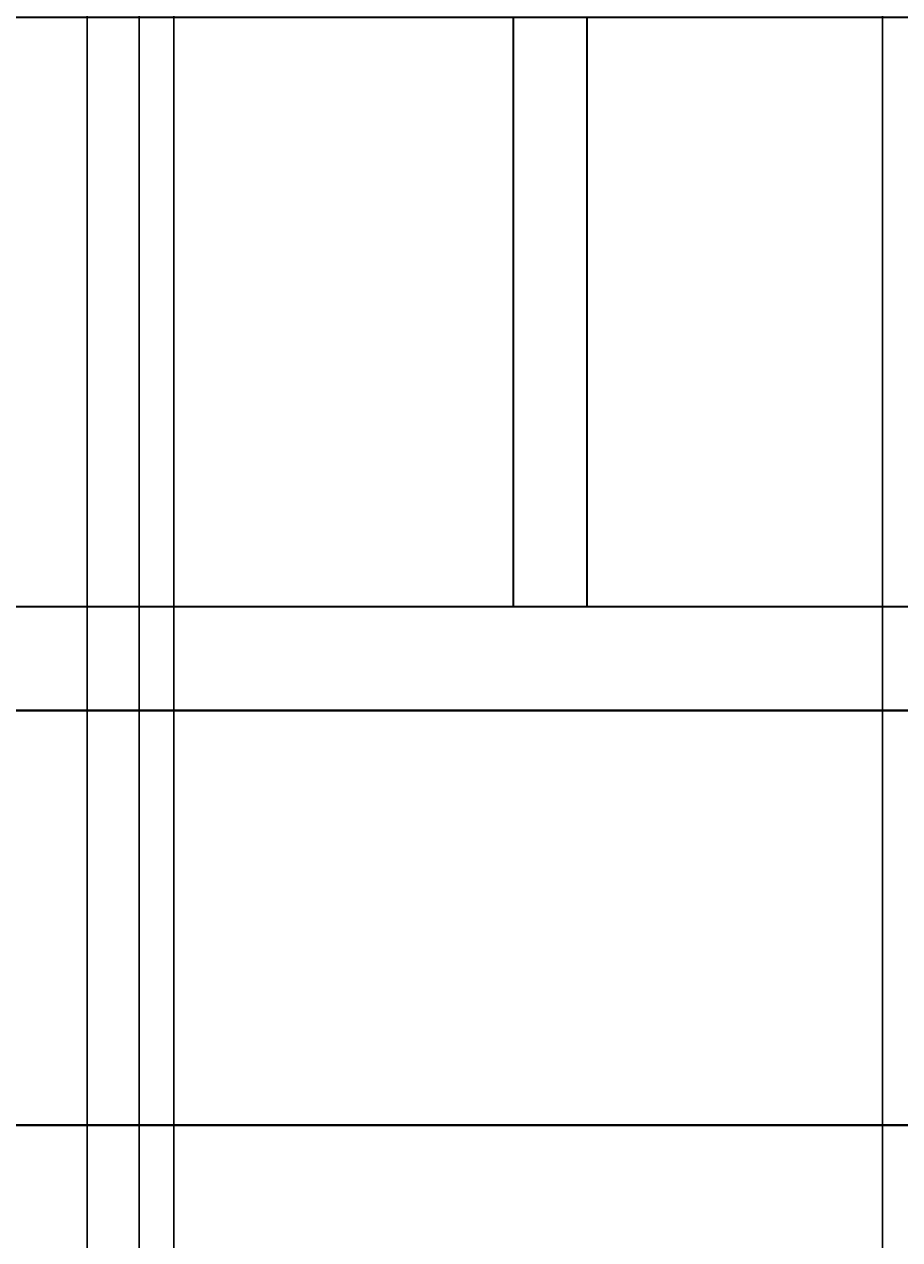
# Model space of a CAD drawing. Units: inches. Extents: x -6 to 289, y -8 to 323.
# Tile 62 of 107: x 186 to 212, y 124 to 159. Entities that reach past the tile are written whole.
import ezdxf

# ---------------------------------------------------------------- set-up
doc = ezdxf.new("R2010")
doc.units = ezdxf.units.IN
doc.header["$MEASUREMENT"] = 0
doc.layers.add('A-ANNO-DIMS', color=2, linetype='Continuous', lineweight=18)
doc.layers.add('A-ELEV', color=7, linetype='Continuous', lineweight=35)
doc.styles.get("Standard").update_dxf_attribs({"font": 'arial.ttf'})
doc.dimstyles.get("Standard").update_dxf_attribs({"dimtxt": 0.18, "dimasz": 0.18, "dimexe": 0.18, "dimexo": 0.0625, "dimgap": 0.09, "dimtad": 0, "dimtih": 1, "dimtoh": 1, "dimdec": 4, "dimzin": 0, "dimdsep": 46, "dimtxsty": 'Standard', "dimcen": 0.09, "dimadec": 0, "dimazin": 0, "dimtfac": 1, "dimtdec": 4, "dimtofl": 0, "dimtmove": 0, "dimatfit": 3, "dimfxl": 1, "dimtolj": 1, "dimtzin": 0, "dimarcsym": 0})

# ---------------------------------------------------------------- blocks, each defined once
blk = doc.blocks.new('*D24')
at = {"layer": 'A-ANNO-DIMS', "color": 0, "lineweight": -2, "transparency": 16777216}
for p, q in [((126.946, 178.654), (288.653, 178.654)), ((288.473, 178.474), (288.473, 159.153)), ((288.473, 139.469), (288.473, 158.789)), ((259.226, 139.289), (288.653, 139.289))]:
    blk.add_line(p, q, dxfattribs=at)
at = {"layer": 'A-ANNO-DIMS', "color": 0, "transparency": 16777216}
for points in [[(288.443, 178.474), (288.503, 178.474), (288.473, 178.654)], [(288.443, 139.469), (288.503, 139.469), (288.473, 139.289)]]:
    blk.add_solid(points, dxfattribs=at)
at = {"layer": 'Defpoints', "color": 0, "transparency": 16777216}
for p in [(126.883, 178.654), (288.473, 178.654), (259.164, 139.289)]:
    blk.add_point(p, dxfattribs=at)
at = {"layer": 'A-ANNO-DIMS', "color": 0, "transparency": 16777216, "insert": (288.473, 158.971), "char_height": 0.18, "attachment_point": 5}
blk.add_mtext('\\A1;39.365', dxfattribs=at)
blk = doc.blocks.new('*D40')
at = {"layer": 'A-ANNO-DIMS', "color": 0, "lineweight": -2, "transparency": 16777216}
for p, q in [((188.292, 226.826), (188.292, -8.391)), ((189.792, 225.326), (189.792, -8.391)), ((188.472, -8.211), (188.796, -8.211)), ((189.612, -8.211), (189.288, -8.211))]:
    blk.add_line(p, q, dxfattribs=at)
at = {"layer": 'A-ANNO-DIMS', "color": 0, "transparency": 16777216}
for points in [[(188.472, -8.181), (188.472, -8.241), (188.292, -8.211)], [(189.612, -8.181), (189.612, -8.241), (189.792, -8.211)]]:
    blk.add_solid(points, dxfattribs=at)
at = {"layer": 'Defpoints', "color": 0, "transparency": 16777216}
for p in [(188.292, 226.889), (189.792, 225.389), (189.792, -8.211)]:
    blk.add_point(p, dxfattribs=at)
at = {"layer": 'A-ANNO-DIMS', "color": 0, "transparency": 16777216, "insert": (189.042, -8.211), "char_height": 0.18, "attachment_point": 5}
blk.add_mtext('\\A1;1.5', dxfattribs=at)
blk = doc.blocks.new('*D41')
at = {"layer": 'A-ANNO-DIMS', "color": 0, "lineweight": -2, "transparency": 16777216}
for p, q in [((189.792, 225.326), (189.792, -8.391)), ((190.792, 224.326), (190.792, -8.391)), ((189.972, -8.211), (190.169, -8.211)), ((190.612, -8.211), (190.415, -8.211))]:
    blk.add_line(p, q, dxfattribs=at)
at = {"layer": 'A-ANNO-DIMS', "color": 0, "transparency": 16777216}
for points in [[(189.972, -8.181), (189.972, -8.241), (189.792, -8.211)], [(190.612, -8.181), (190.612, -8.241), (190.792, -8.211)]]:
    blk.add_solid(points, dxfattribs=at)
at = {"layer": 'Defpoints', "color": 0, "transparency": 16777216}
for p in [(189.792, 225.389), (190.792, 224.389), (190.792, -8.211)]:
    blk.add_point(p, dxfattribs=at)
at = {"layer": 'A-ANNO-DIMS', "color": 0, "transparency": 16777216, "insert": (190.292, -8.211), "char_height": 0.18, "attachment_point": 5}
blk.add_mtext('\\A1;1', dxfattribs=at)
blk = doc.blocks.new('*D42')
at = {"layer": 'A-ANNO-DIMS', "color": 0, "lineweight": -2, "transparency": 16777216}
for p, q in [((190.792, 224.326), (190.792, -8.391)), ((211.292, 224.326), (211.292, -8.391)), ((190.972, -8.211), (200.716, -8.211)), ((211.112, -8.211), (201.368, -8.211))]:
    blk.add_line(p, q, dxfattribs=at)
at = {"layer": 'A-ANNO-DIMS', "color": 0, "transparency": 16777216}
for points in [[(190.972, -8.181), (190.972, -8.241), (190.792, -8.211)], [(211.112, -8.181), (211.112, -8.241), (211.292, -8.211)]]:
    blk.add_solid(points, dxfattribs=at)
at = {"layer": 'Defpoints', "color": 0, "transparency": 16777216}
for p in [(190.792, 224.389), (211.292, 224.389), (211.292, -8.211)]:
    blk.add_point(p, dxfattribs=at)
at = {"layer": 'A-ANNO-DIMS', "color": 0, "transparency": 16777216, "insert": (201.042, -8.211), "char_height": 0.18, "attachment_point": 5}
blk.add_mtext('\\A1;20.5', dxfattribs=at)
blk = doc.blocks.new('*D43')
at = {"layer": 'A-ANNO-DIMS', "color": 0, "lineweight": -2, "transparency": 16777216}
for p, q in [((211.292, 224.326), (211.292, -8.391)), ((212.292, 224.326), (212.292, -8.391)), ((211.472, -8.211), (211.669, -8.211)), ((212.112, -8.211), (211.915, -8.211))]:
    blk.add_line(p, q, dxfattribs=at)
at = {"layer": 'A-ANNO-DIMS', "color": 0, "transparency": 16777216}
for points in [[(211.472, -8.181), (211.472, -8.241), (211.292, -8.211)], [(212.112, -8.181), (212.112, -8.241), (212.292, -8.211)]]:
    blk.add_solid(points, dxfattribs=at)
at = {"layer": 'Defpoints', "color": 0, "transparency": 16777216}
for p in [(211.292, 224.389), (212.292, 224.389), (212.292, -8.211)]:
    blk.add_point(p, dxfattribs=at)
at = {"layer": 'A-ANNO-DIMS', "color": 0, "transparency": 16777216, "insert": (211.792, -8.211), "char_height": 0.18, "attachment_point": 5}
blk.add_mtext('\\A1;1', dxfattribs=at)
blk = doc.blocks.new('*D79')
at = {"layer": 'A-ANNO-DIMS', "color": 0, "lineweight": -2, "transparency": 16777216}
for p, q in [((171.296, 118.033), (171.296, 322.969)), ((188.292, 116.842), (188.292, 322.969)), ((171.476, 322.789), (179.339, 322.789)), ((188.112, 322.789), (180.249, 322.789))]:
    blk.add_line(p, q, dxfattribs=at)
at = {"layer": 'A-ANNO-DIMS', "color": 0, "transparency": 16777216}
for points in [[(171.476, 322.819), (171.476, 322.759), (171.296, 322.789)], [(188.112, 322.819), (188.112, 322.759), (188.292, 322.789)]]:
    blk.add_solid(points, dxfattribs=at)
at = {"layer": 'Defpoints', "color": 0, "transparency": 16777216}
for p in [(188.292, 322.789), (171.296, 117.971), (188.292, 116.779)]:
    blk.add_point(p, dxfattribs=at)
at = {"layer": 'A-ANNO-DIMS', "color": 0, "transparency": 16777216, "insert": (179.794, 322.789), "char_height": 0.18, "attachment_point": 5}
blk.add_mtext('\\A1;16.996', dxfattribs=at)
blk = doc.blocks.new('*D80')
at = {"layer": 'A-ANNO-DIMS', "color": 0, "lineweight": -2, "transparency": 16777216}
for p, q in [((188.292, 116.842), (188.292, 322.969)), ((230.292, 116.842), (230.292, 322.969)), ((188.472, 322.789), (209.07, 322.789)), ((230.112, 322.789), (209.513, 322.789))]:
    blk.add_line(p, q, dxfattribs=at)
at = {"layer": 'A-ANNO-DIMS', "color": 0, "transparency": 16777216}
for points in [[(188.472, 322.819), (188.472, 322.759), (188.292, 322.789)], [(230.112, 322.819), (230.112, 322.759), (230.292, 322.789)]]:
    blk.add_solid(points, dxfattribs=at)
at = {"layer": 'Defpoints', "color": 0, "transparency": 16777216}
for p in [(230.292, 322.789), (188.292, 116.779), (230.292, 116.779)]:
    blk.add_point(p, dxfattribs=at)
at = {"layer": 'A-ANNO-DIMS', "color": 0, "transparency": 16777216, "insert": (209.292, 322.789), "char_height": 0.18, "attachment_point": 5}
blk.add_mtext('\\A1;42', dxfattribs=at)

msp = doc.modelspace()

# ---------------------------------------------------------------- linework, layer by layer
at = {"layer": 'A-ELEV'}
for p, q in [((115.1638, 139.2888), (259.1638, 139.2888)), ((259.1638, 127.2888), (115.1638, 127.2888)), ((115.1638, 127.2888), (259.1638, 127.2888))]:
    msp.add_line(p, q, dxfattribs=at)
for points in [[(247.1638, 139.2888), (115.1638, 139.2888), (115.1638, 162.3484), (247.1638, 162.3484)], [(244.1638, 142.2888), (118.1638, 142.2888), (118.1638, 159.3484), (244.1638, 159.3484)], [(200.6162, 159.3484), (202.741, 159.3484), (202.741, 142.2888), (200.6162, 142.2888)]]:
    msp.add_lwpolyline(points, close=True, dxfattribs=at)

# ---------------------------------------------------------------- dimensions: what is measured, and where the dimension line sits
at = {"layer": 'A-ANNO-DIMS'}
for base, p1, p2, override, picture, middle in [((188.2918, 322.7888), (171.296, 117.9706), (188.2918, 116.7795), {"dimdec": 3, "dimlfac": 1, "dimrnd": 0, "dimzin": 0, "dimdsep": 46, "dimlunit": 2}, '*D79', (179.7939, 322.7888)), ((230.2918, 322.7888), (188.2918, 116.7795), (230.2918, 116.7795), {"dimdec": 0, "dimlfac": 1, "dimrnd": 0, "dimzin": 0, "dimdsep": 46, "dimlunit": 2}, '*D80', (209.2918, 322.7888)), ((189.7918, -8.2112), (188.2918, 226.8887), (189.7918, 225.3887), {"dimdec": 1, "dimlfac": 1, "dimrnd": 0, "dimzin": 0, "dimdsep": 46, "dimlunit": 2}, '*D40', (189.0418, -8.2112)), ((190.7918, -8.2112), (189.7918, 225.3887), (190.7918, 224.3887), {"dimdec": 0, "dimlfac": 1, "dimrnd": 0, "dimzin": 0, "dimdsep": 46, "dimlunit": 2}, '*D41', (190.2918, -8.2112)), ((211.2918, -8.2112), (190.7918, 224.3887), (211.2918, 224.3887), {"dimdec": 1, "dimlfac": 1, "dimrnd": 0, "dimzin": 0, "dimdsep": 46, "dimlunit": 2}, '*D42', (201.0418, -8.2112)), ((212.2918, -8.2112), (211.2918, 224.3887), (212.2918, 224.3887), {"dimdec": 0, "dimlfac": 1, "dimrnd": 0, "dimzin": 0, "dimdsep": 46, "dimlunit": 2}, '*D43', (211.7918, -8.2112))]:
    dim = msp.add_linear_dim(base=base, p1=p1, p2=p2, dimstyle='Standard', override=override, dxfattribs=at)
    dim.commit()
    dim.dimension.update_dxf_attribs({"geometry": picture, "text_midpoint": middle})
dim = msp.add_linear_dim(base=(288.4733, 178.654), p1=(259.1638, 139.2888), p2=(126.8835, 178.654), angle=90, dimstyle='Standard', override={"dimdec": 3, "dimlfac": 1, "dimrnd": 0, "dimzin": 0, "dimdsep": 46, "dimlunit": 2}, dxfattribs=at)
dim.commit()
dim.dimension.update_dxf_attribs({"geometry": '*D24', "text_midpoint": (288.4733, 158.9714)})

doc.saveas('drawing.dxf')
